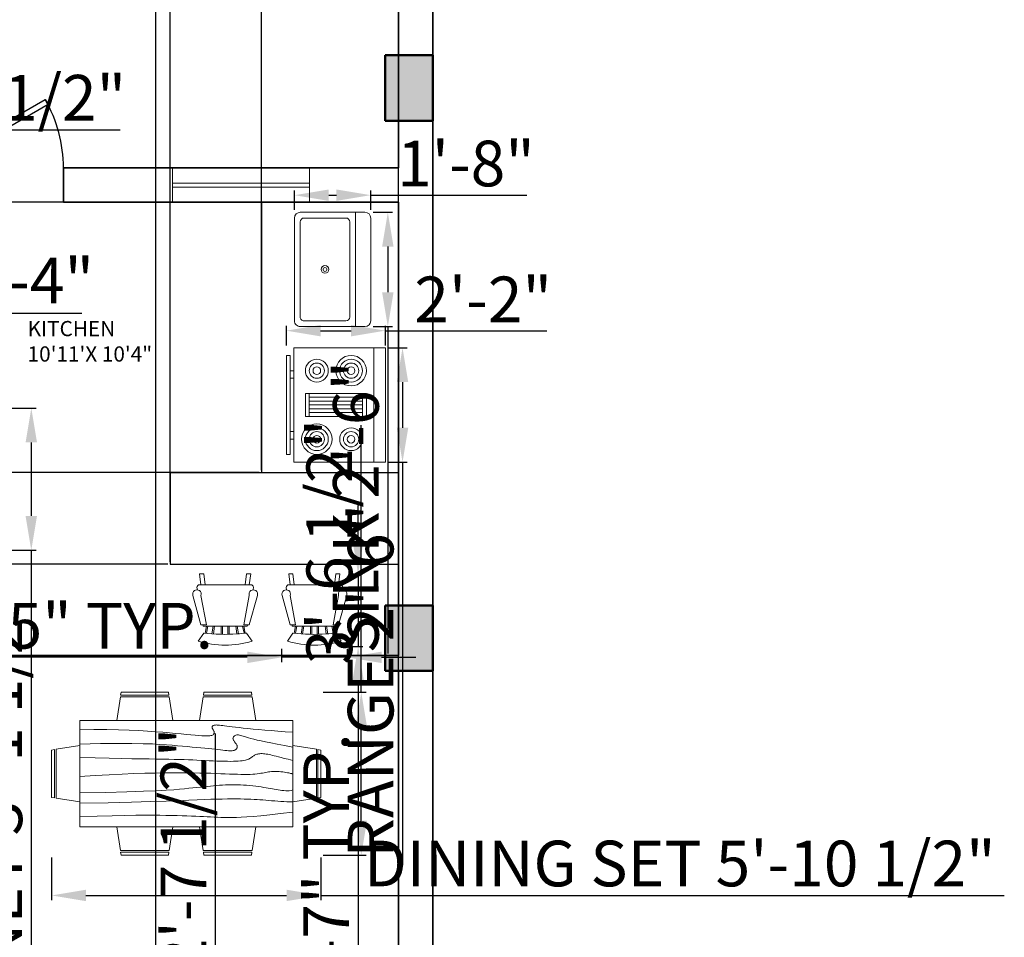
# Model space of a CAD drawing. Units: inches. Extents: x 1132 to 1713, y 3115 to 3781.
# Tile 3 of 4: x 1455 to 1713, y 3365 to 3606. Entities that reach past the tile are written whole.
import ezdxf

# ---------------------------------------------------------------- set-up
doc = ezdxf.new("R2010")
doc.units = ezdxf.units.IN
for name, color, linetype, lineweight in [('A-ANNO-DIMS', 2, 'Continuous', 18), ('A-AREA-IDEN', 7, 'Continuous', 18), ('A-COLS', 1, 'Continuous', 50), ('A-COLS-PATT', 252, 'Continuous', 13), ('A-DOOR', 3, 'Continuous', 25), ('A-EQPM', 8, 'Continuous', 18), ('A-FLOR-CASE', 30, 'Continuous', 25), ('A-FLOR-FIXT', 9, 'Continuous', 18), ('A-FURN', 8, 'Continuous', 18), ('A-GLAZ', 4, 'Continuous', 18), ('A-WALL', 7, 'Continuous', 35)]:
    doc.layers.add(name, color=color, linetype=linetype, lineweight=lineweight)
doc.styles.get("Standard").update_dxf_attribs({"font": 'arial.ttf'})
doc.dimstyles.new('ISO-25', dxfattribs={"dimtxt": 12, "dimasz": 9, "dimexe": 1.25, "dimexo": 0.625, "dimtad": 1, "dimdec": 0, "dimrnd": 2, "dimlunit": 3, "dimtxsty": 'Standard', "dimcen": 2.5, "dimadec": 0, "dimazin": 0, "dimtfac": 1, "dimtdec": 0, "dimtmove": 0, "dimatfit": 3, "dimfxl": 1, "dimarcsym": 0})

# ---------------------------------------------------------------- blocks, each defined once
blk = doc.blocks.new('*U2')
for p, q in [((0, 0), (0, -6)), ((40, 0), (40, -6))]:
    blk.add_line(p, q)
blk.add_lwpolyline([(0, 0), (34.64, 20), (35.52, 18.48), (0.87, -1.52)], close=True)
blk.add_arc((0, 0), 40, 0, 30)
blk = doc.blocks.new('Range-Oven - 30 in top')
for p, q in [((0, -3), (30, -3)), ((12, -6), (18, -6)), ((13, -20), (13, -6)), ((14, -6), (14, -20)), ((15, -20), (15, -6)), ((16, -6), (16, -20)), ((17, -20), (17, -6)), ((18, -20), (12, -20)), ((6, -24), (6, -25)), ((8, -25), (8, -24)), ((22, -25), (22, -24)), ((24, -24), (24, -25))]:
    blk.add_line(p, q)
for points in [[(0, -24), (0, 0), (30, 0), (30, -24)], [(12, -21), (12, -5), (18, -5), (18, -21)], [(2, -26), (2, -25), (28, -25), (28, -26)]]:
    blk.add_lwpolyline(points, close=True)
for centre, radius in [((6, -9), 4), ((6, -9), 3), ((6, -9), 2), ((24, -9), 3), ((24, -9), 2), ((6, -9), 1), ((24, -9), 1), ((6, -18), 3), ((24, -18), 4), ((24, -18), 3), ((6, -18), 2), ((6, -18), 1), ((24, -18), 2), ((24, -18), 1)]:
    blk.add_circle(centre, radius)
blk = doc.blocks.new('Sink-single - 30 in top')
blk.add_line((-15, -3.999996), (15, -3.999996))
for points in [[(-13.5, 0), (13.5, 0)], [(-15, -18.499996), (-15, -1.5)], [(15, -1.5), (15, -18.499996)], [(-13.5, -17.499996), (-13.5, -6.499996)], [(-12.5, -5.499996), (12.5, -5.499996)], [(13.5, -6.499996), (13.5, -17.499996)], [(13.5, -19.999996), (-13.5, -19.999996)], [(12.5, -18.499996), (-12.5, -18.499996)]]:
    blk.add_lwpolyline(points)
for radius in [1, 0.5]:
    blk.add_circle((0, -11.999996), radius)
for centre, radius, start, end in [((-13.5, -1.5), 1.5, 90, 180), ((13.5, -1.5), 1.5, 0, 90), ((-12.5, -6.499996), 1, 90, 180), ((12.5, -6.499996), 1, 0, 90), ((-12.5, -17.499996), 1, 180, 270), ((12.5, -17.499996), 1, 270, 0), ((-13.5, -18.499996), 1.5, 180, 270), ((13.5, -18.499996), 1.5, 270, 0)]:
    blk.add_arc(centre, radius, start, end)
blk = doc.blocks.new('Chair - Rocking')
for p, q in [((-8, -4.5), (-10, -1.5)), ((8, -4.5), (10, -1.5)), ((-8.23428, -6.99939), (-8.3093, -7.47958)), ((-8.23041, -7), (8.23915, -7)), ((-7.5, -4.5), (-7, -7)), ((-6.5, -7), (-7.02225, -4.43)), ((-4.5, -7), (-4.96674, -4.19951)), ((-4, -7), (-4.40532, -4.16272)), ((-1.5, -4.05012), (-1.5, -7)), ((-1, -7), (-1, -4.05012)), ((1, -7), (1, -4.04655)), ((1.5, -4.05012), (1.5, -7)), ((4, -7), (4.40187, -4.18694)), ((4.5, -7), (4.96761, -4.19437)), ((6.5, -7), (7, -4.4057)), ((7.5, -4.5), (7, -7)), ((8.31071, -7.48854), (8.23449, -7.00073)), ((-9, -7.5), (-12, -18.49999)), ((-7, -7.5), (-9, -7.5)), ((-9, -18.49999), (-7, -7.5)), ((7, -7.5), (9, -7.5)), ((9, -18.49999), (7, -7.5)), ((9, -7.5), (12, -18.49999)), ((-10.36644, -20.64523), (-10.5, -21.49999)), ((10.5, -21.49999), (10.3575, -20.58798)), ((-9, -22.49999), (-9.5, -26.49999)), ((0, -22.49999), (-9.5, -22.49999)), ((-8, -26.49999), (-7.5, -22.49999)), ((0, -22.49999), (9.5, -22.49999)), ((8, -26.49999), (7.5, -22.49999)), ((9, -22.49999), (9.5, -26.49999)), ((-9.5, -26.49999), (-8, -26.49999)), ((9.5, -26.49999), (8, -26.49999))]:
    blk.add_line(p, q)
for centre, radius, start, end in [((0, -34.08333), 34.08333, 72.93847, 107.0615), ((0, -68.25004), 64.25, 93.92211, 97.15267), ((0, -68.25004), 64.25, 82.84733, 93.92211), ((-10.5, -18.99999), 1.58114, 161.5651, 18.43495), ((-9.5, -21.49999), 1, 180, 270), ((10.5, -18.99999), 1.58114, 161.5651, 18.43495), ((9.5, -21.49999), 1, 270, 0)]:
    blk.add_arc(centre, radius, start, end)
blk = doc.blocks.new('Dining Set - 36 x 72 in.')
for p, q in [((-22, 27.5), (-22.1562, 26.50042)), ((-22, 27.5), (-6, 27.5)), ((-5.8437, 26.49966), (-6, 27.5)), ((6, 27.5), (5.8438, 26.50042)), ((6, 27.5), (22, 27.5)), ((22.1563, 26.49966), (22, 27.5)), ((-22.2343, 26.00059), (-23.4847, 17.99762)), ((-22.2304, 26), (-5.7608, 26)), ((-5.8416, 26.5), (-22.1534, 26.5)), ((-4.5152, 17.99762), (-5.7655, 25.99926)), ((5.7657, 26.00059), (4.5153, 17.99762)), ((5.7696, 26), (22.2392, 26)), ((22.1584, 26.5), (5.8466, 26.5)), ((23.4848, 17.99762), (22.2345, 25.99926)), ((36, 18), (-36, 18)), ((-36, 18), (-36, -18)), ((36, -18), (36, 18)), ((-45.5, 8), (-44.5004, 8.15617)), ((-45.5, 8), (-45.5, -8)), ((-44.5, -8.15843), (-44.5, 8.15338)), ((-44.0006, 8.23428), (-35.9976, 9.48474)), ((-44, 8.23041), (-44, -8.23915)), ((44.0006, 8.23428), (35.9976, 9.48474)), ((44, 8.23041), (44, -8.23915)), ((44.5, -8.15843), (44.5, 8.15338)), ((45.5, 8), (44.5005, 8.15617)), ((45.5, 8), (45.5, -8)), ((-44.4997, -8.15631), (-45.5, -8)), ((-35.9976, -9.48476), (-43.9993, -8.2345)), ((35.9976, -9.48476), (43.9993, -8.2345)), ((44.4997, -8.15631), (45.5, -8)), ((-36, -18), (36, -18)), ((-22.2343, -26.0006), (-23.4847, -17.99762)), ((-4.5152, -17.99762), (-5.7655, -25.99928)), ((5.7657, -26.0006), (4.5153, -17.99762)), ((23.4848, -17.99762), (22.2345, -25.99928)), ((-22.2304, -26), (-5.7608, -26)), ((-22, -27.5), (-22.1562, -26.50044)), ((-5.8416, -26.5), (-22.1534, -26.5)), ((-5.8437, -26.49967), (-6, -27.5)), ((5.7696, -26), (22.2392, -26)), ((6, -27.5), (5.8438, -26.50044)), ((22.1584, -26.5), (5.8466, -26.5)), ((22.1563, -26.49967), (22, -27.5)), ((-22, -27.5), (-6, -27.5)), ((6, -27.5), (22, -27.5))]:
    blk.add_line(p, q)
for points in [[(-36, 15), (-31.1772, 14.97754), (-26.8079, 14.91406), (-22.8538, 14.81543), (-19.276, 14.6875), (-16.0362, 14.53613), (-13.0957, 14.36718), (-10.4159, 14.18652), (-7.9583, 14), (-5.6904, 13.81315), (-3.6035, 13.63021), (-1.6954, 13.45508), (0.0365, 13.29166), (1.5945, 13.14388), (2.9811, 13.01562), (4.1988, 12.9108), (5.25, 12.83333), (6.1393, 12.78613), (6.8802, 12.76823), (7.4883, 12.77767), (7.9792, 12.8125), (8.3685, 12.87077), (8.6719, 12.95052), (8.9049, 13.0498), (9.0833, 13.16666), (9.2205, 13.29899), (9.3216, 13.44401), (9.3895, 13.59879), (9.4271, 13.76041), (9.4373, 13.92594), (9.4232, 14.09245), (9.3875, 14.257), (9.3333, 14.41666), (9.2638, 14.56917), (9.1836, 14.71484), (9.0975, 14.85465), (9.0104, 14.98958), (8.9272, 15.1206), (8.8529, 15.2487), (8.7922, 15.37483), (8.75, 15.5), (8.7305, 15.62467), (8.7344, 15.74739), (8.7617, 15.86621), (8.8125, 15.97916), (8.8867, 16.08431), (8.9844, 16.17968), (9.1055, 16.26334), (9.25, 16.33333), (9.4189, 16.38802), (9.6172, 16.42708), (9.8506, 16.45052), (10.125, 16.45833), (10.4463, 16.45052), (10.8203, 16.42708), (11.2529, 16.38802), (11.75, 16.33333), (12.3184, 16.26318), (12.9694, 16.17838), (13.7151, 16.07991), (14.5677, 15.96875), (15.5395, 15.84586), (16.6426, 15.71224), (17.8893, 15.56884), (19.2917, 15.41666), (20.859, 15.25667), (22.5879, 15.08984), (24.4721, 14.91715), (26.5052, 14.73958), (28.6809, 14.5581), (30.9929, 14.3737), (33.4347, 14.18733), (36, 14)], [(-36, 10), (-28.9766, 10.14274), (-23.1725, 10.20442), (-18.4241, 10.19775), (-14.5677, 10.13541), (-11.4399, 10.03011), (-8.877, 9.89453), (-6.7154, 9.74137), (-4.7917, 9.58333), (-2.9698, 9.43082), (-1.2246, 9.28515), (0.4415, 9.14534), (2.026, 9.01041), (3.5266, 8.87939), (4.9408, 8.7513), (6.266, 8.62516), (7.5, 8.5), (8.6411, 8.37549), (9.6914, 8.2539), (10.6538, 8.13818), (11.5312, 8.03125), (12.3267, 7.93603), (13.043, 7.85547), (13.6831, 7.79248), (14.25, 7.75), (14.7471, 7.7303), (15.1797, 7.73307), (15.5537, 7.75732), (15.875, 7.80208), (16.1494, 7.86637), (16.3828, 7.94922), (16.5811, 8.04964), (16.75, 8.16666), (16.8944, 8.29915), (17.0143, 8.44531), (17.1089, 8.60319), (17.1771, 8.77083), (17.218, 8.94629), (17.2305, 9.1276), (17.2137, 9.31282), (17.1667, 9.5), (17.0895, 9.6875), (16.987, 9.875), (16.8649, 10.0625), (16.7292, 10.25), (16.5856, 10.4375), (16.4401, 10.625), (16.2985, 10.8125), (16.1667, 11), (16.05, 11.18733), (15.9518, 11.3737), (15.8752, 11.5581), (15.8229, 11.73958), (15.798, 11.91715), (15.8034, 12.08984), (15.842, 12.25667), (15.9167, 12.41666), (16.0295, 12.56836), (16.1784, 12.70833), (16.3605, 12.83268), (16.5729, 12.9375), (16.8127, 13.01888), (17.0768, 13.07291), (17.3625, 13.0957), (17.6667, 13.08333), (17.9894, 13.03312), (18.3418, 12.94726), (18.7382, 12.82918), (19.1927, 12.68229), (19.7195, 12.51001), (20.3327, 12.31575), (21.0465, 12.10294), (21.875, 11.875), (22.8357, 11.63354), (23.959, 11.37304), (25.2786, 11.08618), (26.8282, 10.76562), (28.6414, 10.40405), (30.752, 9.99414), (33.1936, 9.52856), (36, 9)], [(-36, 5.5), (-30.7157, 5.3348), (-26.069, 5.20963), (-21.9946, 5.11767), (-18.4271, 5.05208), (-15.3009, 5.00602), (-12.5508, 4.97265), (-10.1112, 4.94515), (-7.9167, 4.91666), (-5.909, 4.88167), (-4.0586, 4.83984), (-2.3429, 4.79215), (-0.7396, 4.73958), (0.7739, 4.6831), (2.22, 4.6237), (3.6213, 4.56233), (5, 4.5), (6.373, 4.43782), (7.7344, 4.3776), (9.0723, 4.32129), (10.375, 4.27083), (11.6309, 4.22819), (12.8281, 4.19531), (13.9551, 4.17415), (15, 4.16666), (15.954, 4.17448), (16.819, 4.19791), (17.6001, 4.23698), (18.3021, 4.29166), (18.9299, 4.36198), (19.4883, 4.44791), (19.9823, 4.54948), (20.4167, 4.66666), (20.7969, 4.79899), (21.1302, 4.94401), (21.4245, 5.09879), (21.6875, 5.26041), (21.9271, 5.42594), (22.1511, 5.59245), (22.3672, 5.757), (22.5834, 5.91666), (22.8065, 6.06868), (23.0404, 6.21093), (23.2879, 6.34147), (23.5521, 6.45833), (23.8358, 6.55957), (24.142, 6.64323), (24.4735, 6.70735), (24.8334, 6.75), (25.2235, 6.76969), (25.642, 6.76692), (26.0858, 6.74267), (26.5521, 6.69791), (27.0379, 6.63362), (27.5404, 6.55078), (28.0565, 6.45036), (28.5834, 6.33333), (29.1242, 6.19987), (29.7071, 6.04687), (30.3661, 5.87044), (31.1354, 5.66666), (32.0493, 5.43164), (33.142, 5.16146), (34.4475, 4.85221), (36, 4.5)], [(-36, -1), (-30.7915, -0.6591), (-26.0195, -0.38216), (-21.6519, -0.16284), (-17.6563, 0.00521), (-14.0005, 0.12833), (-10.6523, 0.21289), (-7.5796, 0.26522), (-4.75, 0.29166), (-2.134, 0.29793), (0.2878, 0.28711), (2.5317, 0.26163), (4.6146, 0.22396), (6.5529, 0.17651), (8.3633, 0.12174), (10.0623, 0.06209), (11.6667, 0), (13.1899, -0.06201), (14.6341, -0.1211), (15.9982, -0.17432), (17.2813, -0.21875), (18.4823, -0.25147), (19.6003, -0.26953), (20.6343, -0.27002), (21.5834, -0.25), (22.4481, -0.20768), (23.2357, -0.14584), (23.9549, -0.06836), (24.6146, 0.02083), (25.2235, 0.11784), (25.7904, 0.21875), (26.3241, 0.31966), (26.8334, 0.41666), (27.3265, 0.50618), (27.8099, 0.58593), (28.2894, 0.65397), (28.7709, 0.70833), (29.2601, 0.74707), (29.763, 0.76823), (30.2855, 0.76985), (30.8334, 0.75), (31.4088, 0.70784), (31.9994, 0.64713), (32.589, 0.57275), (33.1615, 0.48958), (33.7008, 0.4025), (34.1908, 0.3164), (34.6153, 0.23616), (34.9584, 0.16666), (35.2099, 0.11165), (35.3848, 0.07031), (35.504, 0.04069), (35.5886, 0.02083), (35.6594, 0.00879), (35.7377, 0.0026), (35.8442, 0.00032), (36, 0)], [(-36, -6.5), (-27.1843, -6.31267), (-20.084, -6.1263), (-14.469, -5.9419), (-10.1094, -5.76042), (-6.7752, -5.58285), (-4.2363, -5.41016), (-2.2629, -5.24333), (-0.625, -5.08334), (0.8708, -4.93099), (2.2715, -4.78646), (3.5872, -4.64974), (4.8281, -4.52084), (6.0046, -4.39974), (7.127, -4.28646), (8.2053, -4.18099), (9.25, -4.08334), (10.2705, -3.99382), (11.2734, -3.91407), (12.2647, -3.84603), (13.25, -3.79167), (14.2354, -3.75293), (15.2266, -3.73177), (16.2295, -3.73015), (17.25, -3.75), (18.2912, -3.79248), (19.3451, -3.85547), (20.4009, -3.93604), (21.4479, -4.03125), (22.4754, -4.13819), (23.4727, -4.25391), (24.4289, -4.37549), (25.3334, -4.5), (26.1785, -4.62492), (26.9694, -4.74935), (27.7145, -4.87281), (28.4219, -4.99479), (29.1, -5.11483), (29.7572, -5.23242), (30.4016, -5.34709), (31.0417, -5.45834), (31.6837, -5.56437), (32.3262, -5.65821), (32.9658, -5.73153), (33.599, -5.77604), (34.2224, -5.78345), (34.8327, -5.74545), (35.4264, -5.65373), (36, -5.5)], [(-36, -10), (-26.4022, -9.81299), (-18.4675, -9.62891), (-11.9839, -9.45069), (-6.7396, -9.28125), (-2.5226, -9.12354), (0.8789, -8.98047), (3.6769, -8.85498), (6.0833, -8.75), (8.2767, -8.66765), (10.3021, -8.60677), (12.1712, -8.56543), (13.8958, -8.54167), (15.4876, -8.53353), (16.9583, -8.53907), (18.3197, -8.55632), (19.5834, -8.58334), (20.7616, -8.61841), (21.8685, -8.66081), (22.9188, -8.71004), (23.9271, -8.76563), (24.9081, -8.82707), (25.8763, -8.89388), (26.8465, -8.96558), (27.8334, -9.04167), (28.8474, -9.12118), (29.8828, -9.20117), (30.93, -9.27824), (31.9792, -9.34896), (33.0205, -9.40991), (34.0443, -9.45768), (35.0407, -9.48885), (36, -9.5)], [(-36, -14.5), (-30.0881, -14.33513), (-25.0332, -14.21224), (-20.7312, -14.12647), (-17.0781, -14.07292), (-13.97, -14.04671), (-11.3027, -14.04297), (-8.9724, -14.05681), (-6.875, -14.08334), (-4.9224, -14.11833), (-3.0905, -14.16016), (-1.3709, -14.20785), (0.2448, -14.26042), (1.7647, -14.3169), (3.1973, -14.3763), (4.5507, -14.43767), (5.8333, -14.5), (7.0554, -14.5621), (8.235, -14.62175), (9.3922, -14.67652), (10.5469, -14.72396), (11.7192, -14.76164), (12.929, -14.78711), (14.1965, -14.79794), (15.5417, -14.79167), (16.9933, -14.76424), (18.6152, -14.70508), (20.4804, -14.60197), (22.6615, -14.44271), (25.2312, -14.21509), (28.2624, -13.9069), (31.8277, -13.50594), (36, -13)]]:
    blk.add_lwpolyline(points)
blk = doc.blocks.new('WIN-36IN')
for p, q in [((-36, 0), (-36, 9)), ((-36, 9), (0, 9)), ((0, 9), (0, 0)), ((-36, 5), (0, 5)), ((0, 4), (-36, 4)), ((0, 0), (-36, 0))]:
    blk.add_line(p, q)
blk = doc.blocks.new('*D23')
at = {"layer": 'A-ANNO-DIMS', "color": 0, "lineweight": -2, "transparency": 16777216}
for p, q in [((1386.32, 3573.51), (1386.32, 3578.18)), ((1410.75, 3573.51), (1410.75, 3578.18)), ((1395.32, 3576.93), (1401.75, 3576.93)), ((1410.75, 3576.93), (1481.07, 3576.93))]:
    blk.add_line(p, q, dxfattribs=at)
at = {"layer": 'A-ANNO-DIMS', "color": 0, "transparency": 16777216}
for points in [[(1395.32, 3578.43), (1395.32, 3575.43), (1386.32, 3576.93)], [(1401.75, 3578.43), (1401.75, 3575.43), (1410.75, 3576.93)]]:
    blk.add_solid(points, dxfattribs=at)
at = {"layer": 'Defpoints', "color": 0, "transparency": 16777216}
for p in [(1410.75, 3576.93), (1386.32, 3572.88), (1410.75, 3572.88)]:
    blk.add_point(p, dxfattribs=at)
at = {"layer": 'A-ANNO-DIMS', "color": 0, "transparency": 16777216, "insert": (1450.41, 3583.76), "char_height": 12, "attachment_point": 5}
blk.add_mtext('2\'-0 1/2"', dxfattribs=at)
blk = doc.blocks.new('*D24')
at = {"layer": 'A-ANNO-DIMS', "color": 0, "lineweight": -2, "transparency": 16777216}
for p, q in [((1543.52, 3469.28), (1543.52, 3478.28)), ((1541.29, 3460.28), (1544.77, 3460.28)), ((1543.52, 3460.28), (1543.52, 3441.25)), ((1541.29, 3441.25), (1544.77, 3441.25)), ((1543.52, 3432.25), (1543.52, 3273.09))]:
    blk.add_line(p, q, dxfattribs=at)
at = {"layer": 'A-ANNO-DIMS', "color": 0, "transparency": 16777216}
for points in [[(1542.02, 3469.28), (1545.02, 3469.28), (1543.52, 3460.28)], [(1542.02, 3432.25), (1545.02, 3432.25), (1543.52, 3441.25)]]:
    blk.add_solid(points, dxfattribs=at)
at = {"layer": 'Defpoints', "color": 0, "transparency": 16777216}
for p in [(1540.66, 3460.28), (1540.66, 3441.25), (1543.52, 3441.25)]:
    blk.add_point(p, dxfattribs=at)
at = {"layer": 'A-ANNO-DIMS', "color": 0, "transparency": 16777216, "insert": (1536.68, 3348.17), "char_height": 12, "attachment_point": 5, "rotation": 90}
blk.add_mtext('ROCKER 1\'-7" TYP.', dxfattribs=at)
blk = doc.blocks.new('*D25')
at = {"layer": 'A-ANNO-DIMS', "color": 0, "lineweight": -2, "transparency": 16777216}
for p, q in [((1514.43, 3438.39), (1432.17, 3438.39)), ((1523.43, 3440.62), (1523.43, 3437.14)), ((1540.66, 3438.39), (1523.43, 3438.39)), ((1540.66, 3440.62), (1540.66, 3437.14)), ((1549.66, 3438.39), (1558.66, 3438.39))]:
    blk.add_line(p, q, dxfattribs=at)
at = {"layer": 'A-ANNO-DIMS', "color": 0, "transparency": 16777216}
for points in [[(1514.43, 3439.89), (1514.43, 3436.89), (1523.43, 3438.39)], [(1549.66, 3439.89), (1549.66, 3436.89), (1540.66, 3438.39)]]:
    blk.add_solid(points, dxfattribs=at)
at = {"layer": 'Defpoints', "color": 0, "transparency": 16777216}
for p in [(1523.43, 3441.25), (1540.66, 3441.25), (1523.43, 3438.39)]:
    blk.add_point(p, dxfattribs=at)
at = {"layer": 'A-ANNO-DIMS', "color": 0, "transparency": 16777216, "insert": (1468.8, 3445.14), "char_height": 12, "attachment_point": 5}
blk.add_mtext('1\'-5" TYP.', dxfattribs=at)
blk = doc.blocks.new('*D31')
at = {"layer": 'A-ANNO-DIMS', "color": 0, "lineweight": -2, "transparency": 16777216}
for p, q in [((1506.04, 3348.05), (1506.04, 3418.37)), ((1498.97, 3348.05), (1507.29, 3348.05)), ((1506.04, 3325.7), (1506.04, 3339.05)), ((1498.97, 3316.7), (1507.29, 3316.7))]:
    blk.add_line(p, q, dxfattribs=at)
at = {"layer": 'A-ANNO-DIMS', "color": 0, "transparency": 16777216}
for points in [[(1504.54, 3339.05), (1507.54, 3339.05), (1506.04, 3348.05)], [(1504.54, 3325.7), (1507.54, 3325.7), (1506.04, 3316.7)]]:
    blk.add_solid(points, dxfattribs=at)
at = {"layer": 'Defpoints', "color": 0, "transparency": 16777216}
for p in [(1498.35, 3348.05), (1506.04, 3348.05), (1498.35, 3316.7)]:
    blk.add_point(p, dxfattribs=at)
at = {"layer": 'A-ANNO-DIMS', "color": 0, "transparency": 16777216, "insert": (1499.21, 3387.71), "char_height": 12, "attachment_point": 5, "rotation": 90}
blk.add_mtext('2\'-7 1/2"', dxfattribs=at)
blk = doc.blocks.new('*D34')
at = {"layer": 'A-ANNO-DIMS', "color": 0, "lineweight": -2, "transparency": 16777216}
for p, q in [((1551.3, 3519.66), (1556.43, 3519.66)), ((1555.18, 3510.66), (1555.18, 3498.66)), ((1551.3, 3489.66), (1556.43, 3489.66)), ((1555.18, 3489.66), (1555.18, 3383.86))]:
    blk.add_line(p, q, dxfattribs=at)
at = {"layer": 'A-ANNO-DIMS', "color": 0, "transparency": 16777216}
for points in [[(1553.68, 3510.66), (1556.68, 3510.66), (1555.18, 3519.66)], [(1553.68, 3498.66), (1556.68, 3498.66), (1555.18, 3489.66)]]:
    blk.add_solid(points, dxfattribs=at)
at = {"layer": 'Defpoints', "color": 0, "transparency": 16777216}
for p in [(1550.68, 3519.66), (1550.68, 3489.66), (1555.18, 3489.66)]:
    blk.add_point(p, dxfattribs=at)
at = {"layer": 'A-ANNO-DIMS', "color": 0, "transparency": 16777216, "insert": (1548.35, 3432.26), "char_height": 12, "attachment_point": 5, "rotation": 90}
blk.add_mtext('RANGE 2\'-6"', dxfattribs=at)
blk = doc.blocks.new('*D35')
at = {"layer": 'A-ANNO-DIMS', "color": 0, "lineweight": -2, "transparency": 16777216}
for p, q in [((1524.68, 3520.28), (1524.68, 3525.41)), ((1533.68, 3524.16), (1541.68, 3524.16)), ((1550.68, 3520.28), (1550.68, 3525.41)), ((1550.68, 3524.16), (1593.03, 3524.16))]:
    blk.add_line(p, q, dxfattribs=at)
at = {"layer": 'A-ANNO-DIMS', "color": 0, "transparency": 16777216}
for points in [[(1533.68, 3525.66), (1533.68, 3522.66), (1524.68, 3524.16)], [(1541.68, 3525.66), (1541.68, 3522.66), (1550.68, 3524.16)]]:
    blk.add_solid(points, dxfattribs=at)
at = {"layer": 'Defpoints', "color": 0, "transparency": 16777216}
for p in [(1550.68, 3524.16), (1524.68, 3519.66), (1550.68, 3519.66)]:
    blk.add_point(p, dxfattribs=at)
at = {"layer": 'A-ANNO-DIMS', "color": 0, "transparency": 16777216, "insert": (1576.35, 3530.81), "char_height": 12, "attachment_point": 5}
blk.add_mtext('2\'-2"', dxfattribs=at)
blk = doc.blocks.new('*D40')
at = {"layer": 'A-ANNO-DIMS', "color": 0, "lineweight": -2, "transparency": 16777216}
for p, q in [((1452.73, 3503.82), (1458.96, 3503.82)), ((1457.71, 3494.82), (1457.71, 3475.51)), ((1452.73, 3466.51), (1458.96, 3466.51)), ((1457.71, 3466.51), (1457.71, 3319.22))]:
    blk.add_line(p, q, dxfattribs=at)
at = {"layer": 'A-ANNO-DIMS', "color": 0, "transparency": 16777216}
for points in [[(1456.21, 3494.82), (1459.21, 3494.82), (1457.71, 3503.82)], [(1456.21, 3475.51), (1459.21, 3475.51), (1457.71, 3466.51)]]:
    blk.add_solid(points, dxfattribs=at)
at = {"layer": 'Defpoints', "color": 0, "transparency": 16777216}
for p in [(1452.11, 3503.82), (1452.11, 3466.51), (1457.71, 3466.51)]:
    blk.add_point(p, dxfattribs=at)
at = {"layer": 'A-ANNO-DIMS', "color": 0, "transparency": 16777216, "insert": (1450.87, 3388.36), "char_height": 12, "attachment_point": 5, "rotation": 90}
blk.add_mtext('CABINET 3\'-1 1/2"', dxfattribs=at)
blk = doc.blocks.new('*D42')
at = {"layer": 'A-ANNO-DIMS', "color": 0, "lineweight": -2, "transparency": 16777216}
for p, q in [((1547.44, 3555.24), (1552.57, 3555.24)), ((1551.32, 3546.24), (1551.32, 3534.24)), ((1547.44, 3525.24), (1552.57, 3525.24)), ((1551.32, 3525.24), (1551.32, 3439.37))]:
    blk.add_line(p, q, dxfattribs=at)
at = {"layer": 'A-ANNO-DIMS', "color": 0, "transparency": 16777216}
for points in [[(1549.82, 3546.24), (1552.82, 3546.24), (1551.32, 3555.24)], [(1549.82, 3534.24), (1552.82, 3534.24), (1551.32, 3525.24)]]:
    blk.add_solid(points, dxfattribs=at)
at = {"layer": 'Defpoints', "color": 0, "transparency": 16777216}
for p in [(1546.82, 3555.24), (1546.82, 3525.24), (1551.32, 3525.24)]:
    blk.add_point(p, dxfattribs=at)
at = {"layer": 'A-ANNO-DIMS', "color": 0, "transparency": 16777216, "insert": (1544.49, 3477.81), "char_height": 12, "attachment_point": 5, "rotation": 90}
blk.add_mtext('SINK 2\'-6"', dxfattribs=at)
blk = doc.blocks.new('*D43')
at = {"layer": 'A-ANNO-DIMS', "color": 0, "lineweight": -2, "transparency": 16777216}
for p, q in [((1526.82, 3555.87), (1526.82, 3560.99)), ((1535.82, 3559.74), (1537.82, 3559.74)), ((1546.82, 3555.87), (1546.82, 3560.99)), ((1546.82, 3559.74), (1587.84, 3559.74))]:
    blk.add_line(p, q, dxfattribs=at)
at = {"layer": 'A-ANNO-DIMS', "color": 0, "transparency": 16777216}
for points in [[(1535.82, 3561.24), (1535.82, 3558.24), (1526.82, 3559.74)], [(1537.82, 3561.24), (1537.82, 3558.24), (1546.82, 3559.74)]]:
    blk.add_solid(points, dxfattribs=at)
at = {"layer": 'Defpoints', "color": 0, "transparency": 16777216}
for p in [(1546.82, 3559.74), (1526.82, 3555.24), (1546.82, 3555.24)]:
    blk.add_point(p, dxfattribs=at)
at = {"layer": 'A-ANNO-DIMS', "color": 0, "transparency": 16777216, "insert": (1571.83, 3566.5), "char_height": 12, "attachment_point": 5}
blk.add_mtext('1\'-8"', dxfattribs=at)
blk = doc.blocks.new('*D44')
at = {"layer": 'A-ANNO-DIMS', "color": 0, "lineweight": -2, "transparency": 16777216}
for p, q in [((1463.04, 3385.85), (1463.04, 3374.62)), ((1533.74, 3385.85), (1533.74, 3374.62)), ((1472.04, 3375.87), (1524.74, 3375.87)), ((1533.74, 3375.87), (1713.17, 3375.87))]:
    blk.add_line(p, q, dxfattribs=at)
at = {"layer": 'A-ANNO-DIMS', "color": 0, "transparency": 16777216}
for points in [[(1472.04, 3377.37), (1472.04, 3374.37), (1463.04, 3375.87)], [(1524.74, 3377.37), (1524.74, 3374.37), (1533.74, 3375.87)]]:
    blk.add_solid(points, dxfattribs=at)
at = {"layer": 'Defpoints', "color": 0, "transparency": 16777216}
for p in [(1463.04, 3386.48), (1533.74, 3386.48), (1533.74, 3375.87)]:
    blk.add_point(p, dxfattribs=at)
at = {"layer": 'A-ANNO-DIMS', "color": 0, "transparency": 16777216, "insert": (1627.96, 3382.7), "char_height": 12, "attachment_point": 5}
blk.add_mtext('DINING SET 5\'-10 1/2"', dxfattribs=at)
blk = doc.blocks.new('*D45')
at = {"layer": 'A-ANNO-DIMS', "color": 0, "lineweight": -2, "transparency": 16777216}
for p, q in [((1544.35, 3429.21), (1544.35, 3499.31)), ((1534.37, 3429.21), (1545.6, 3429.21)), ((1544.35, 3395.48), (1544.35, 3420.21)), ((1534.37, 3386.48), (1545.6, 3386.48))]:
    blk.add_line(p, q, dxfattribs=at)
at = {"layer": 'A-ANNO-DIMS', "color": 0, "transparency": 16777216}
for points in [[(1542.85, 3420.21), (1545.85, 3420.21), (1544.35, 3429.21)], [(1542.85, 3395.48), (1545.85, 3395.48), (1544.35, 3386.48)]]:
    blk.add_solid(points, dxfattribs=at)
at = {"layer": 'Defpoints', "color": 0, "transparency": 16777216}
for p in [(1533.74, 3429.21), (1544.35, 3429.21), (1533.74, 3386.48)]:
    blk.add_point(p, dxfattribs=at)
at = {"layer": 'A-ANNO-DIMS', "color": 0, "transparency": 16777216, "insert": (1537.51, 3468.76), "char_height": 12, "attachment_point": 5, "rotation": 90}
blk.add_mtext('3\'-6 1/2"', dxfattribs=at)
blk = doc.blocks.new('*D50')
at = {"layer": 'A-ANNO-DIMS', "color": 0, "lineweight": -2, "transparency": 16777216}
for p, q in [((1490.38, 3260.74), (1490.38, 3701.81)), ((1554.16, 3217.5), (1554.16, 3701.81)), ((1499.38, 3700.56), (1545.16, 3700.56))]:
    blk.add_line(p, q, dxfattribs=at)
at = {"layer": 'A-ANNO-DIMS', "color": 0, "transparency": 16777216}
for points in [[(1499.38, 3702.06), (1499.38, 3699.06), (1490.38, 3700.56)], [(1545.16, 3702.06), (1545.16, 3699.06), (1554.16, 3700.56)]]:
    blk.add_solid(points, dxfattribs=at)
at = {"layer": 'Defpoints', "color": 0, "transparency": 16777216}
for p in [(1554.16, 3700.56), (1490.38, 3260.12), (1554.16, 3216.88)]:
    blk.add_point(p, dxfattribs=at)
at = {"layer": 'A-ANNO-DIMS', "color": 0, "transparency": 16777216, "insert": (1522.27, 3707.29), "char_height": 12, "attachment_point": 5}
blk.add_mtext('5\'-4"', dxfattribs=at)
blk = doc.blocks.new('*D55')
at = {"layer": 'A-ANNO-DIMS', "color": 0, "lineweight": -2, "transparency": 16777216}
for p, q in [((1494.16, 3463.5), (1494.16, 3701.81)), ((1554.16, 3463.5), (1554.16, 3701.81)), ((1503.16, 3700.56), (1545.16, 3700.56))]:
    blk.add_line(p, q, dxfattribs=at)
at = {"layer": 'A-ANNO-DIMS', "color": 0, "transparency": 16777216}
for points in [[(1503.16, 3702.06), (1503.16, 3699.06), (1494.16, 3700.56)], [(1545.16, 3702.06), (1545.16, 3699.06), (1554.16, 3700.56)]]:
    blk.add_solid(points, dxfattribs=at)
at = {"layer": 'Defpoints', "color": 0, "transparency": 16777216}
for p in [(1554.16, 3700.56), (1494.16, 3462.88), (1554.16, 3462.88)]:
    blk.add_point(p, dxfattribs=at)
at = {"layer": 'A-ANNO-DIMS', "color": 0, "transparency": 16777216, "insert": (1524.16, 3707.31), "char_height": 12, "attachment_point": 5}
blk.add_mtext('5\'-0"', dxfattribs=at)
blk = doc.blocks.new('*D56')
at = {"layer": 'A-ANNO-DIMS', "color": 0, "lineweight": -2, "transparency": 16777216}
for p, q in [((1238.49, 3486.88), (1238.49, 3529.23)), ((1493.53, 3486.88), (1237.24, 3486.88)), ((1238.49, 3471.88), (1238.49, 3477.88)), ((1493.53, 3462.88), (1237.24, 3462.88))]:
    blk.add_line(p, q, dxfattribs=at)
at = {"layer": 'A-ANNO-DIMS', "color": 0, "transparency": 16777216}
for points in [[(1236.99, 3477.88), (1239.99, 3477.88), (1238.49, 3486.88)], [(1236.99, 3471.88), (1239.99, 3471.88), (1238.49, 3462.88)]]:
    blk.add_solid(points, dxfattribs=at)
at = {"layer": 'Defpoints', "color": 0, "transparency": 16777216}
for p in [(1238.49, 3486.88), (1494.16, 3486.88), (1494.16, 3462.88)]:
    blk.add_point(p, dxfattribs=at)
at = {"layer": 'A-ANNO-DIMS', "color": 0, "transparency": 16777216, "insert": (1231.73, 3512.55), "char_height": 12, "attachment_point": 5, "rotation": 90}
blk.add_mtext('2\'-0"', dxfattribs=at)
blk = doc.blocks.new('*D57')
at = {"layer": 'A-ANNO-DIMS', "color": 0, "lineweight": -2, "transparency": 16777216}
for p, q in [((1517.53, 3557.88), (1237.24, 3557.88)), ((1238.49, 3495.88), (1238.49, 3548.88)), ((1517.53, 3486.88), (1237.24, 3486.88))]:
    blk.add_line(p, q, dxfattribs=at)
at = {"layer": 'A-ANNO-DIMS', "color": 0, "transparency": 16777216}
for points in [[(1236.99, 3548.88), (1239.99, 3548.88), (1238.49, 3557.88)], [(1236.99, 3495.88), (1239.99, 3495.88), (1238.49, 3486.88)]]:
    blk.add_solid(points, dxfattribs=at)
at = {"layer": 'Defpoints', "color": 0, "transparency": 16777216}
for p in [(1238.49, 3557.88), (1518.16, 3557.88), (1518.16, 3486.88)]:
    blk.add_point(p, dxfattribs=at)
at = {"layer": 'A-ANNO-DIMS', "color": 0, "transparency": 16777216, "insert": (1231.73, 3522.38), "char_height": 12, "attachment_point": 5, "rotation": 90}
blk.add_mtext('5\'-11"', dxfattribs=at)
blk = doc.blocks.new('*D58')
at = {"layer": 'A-ANNO-DIMS', "color": 0, "lineweight": -2, "transparency": 16777216}
for p, q in [((1494.16, 3487.5), (1494.16, 3701.81)), ((1518.16, 3487.5), (1518.16, 3701.81)), ((1503.16, 3700.56), (1509.16, 3700.56)), ((1518.16, 3700.56), (1560.51, 3700.56))]:
    blk.add_line(p, q, dxfattribs=at)
at = {"layer": 'A-ANNO-DIMS', "color": 0, "transparency": 16777216}
for points in [[(1503.16, 3702.06), (1503.16, 3699.06), (1494.16, 3700.56)], [(1509.16, 3702.06), (1509.16, 3699.06), (1518.16, 3700.56)]]:
    blk.add_solid(points, dxfattribs=at)
at = {"layer": 'Defpoints', "color": 0, "transparency": 16777216}
for p in [(1518.16, 3700.56), (1494.16, 3486.88), (1518.16, 3486.88)]:
    blk.add_point(p, dxfattribs=at)
at = {"layer": 'A-ANNO-DIMS', "color": 0, "transparency": 16777216, "insert": (1543.84, 3707.31), "char_height": 12, "attachment_point": 5}
blk.add_mtext('2\'-0"', dxfattribs=at)
blk = doc.blocks.new('*D59')
at = {"layer": 'A-ANNO-DIMS', "color": 0, "lineweight": -2, "transparency": 16777216}
for p, q in [((1381.6, 3528.66), (1372.6, 3528.66)), ((1390.6, 3528.66), (1406.81, 3528.66)), ((1471.02, 3528.66), (1415.81, 3528.66))]:
    blk.add_line(p, q, dxfattribs=at)
at = {"layer": 'A-ANNO-DIMS', "color": 0, "transparency": 16777216}
for points in [[(1381.6, 3530.16), (1381.6, 3527.16), (1390.6, 3528.66)], [(1415.81, 3530.16), (1415.81, 3527.16), (1406.81, 3528.66)]]:
    blk.add_solid(points, dxfattribs=at)
at = {"layer": 'Defpoints', "color": 0, "transparency": 16777216}
for p in [(1390.6, 3528.66), (1406.81, 3528.66)]:
    blk.add_point(p, dxfattribs=at)
at = {"layer": 'A-ANNO-DIMS', "color": 0, "transparency": 16777216, "insert": (1447.92, 3535.75), "char_height": 12, "attachment_point": 5, "rotation": 0.002}
blk.add_mtext('∅1\'-4"', dxfattribs=at)

msp = doc.modelspace()

# ---------------------------------------------------------------- hatches: boundary and pattern name
at = {"layer": 'A-COLS-PATT'}
h = msp.add_hatch(color=256, dxfattribs=at)
h.dxf.hatch_style = 1
h.paths.add_polyline_path([(1550.64, 3579.3), (1554.16, 3579.3), (1554.16, 3596.47), (1550.64, 3596.47)])
h = msp.add_hatch(color=256, dxfattribs=at)
h.dxf.hatch_style = 1
h.paths.add_polyline_path([(1563.14, 3596.47), (1554.16, 3596.47), (1554.16, 3579.3), (1563.14, 3579.3)])
h = msp.add_hatch(color=256, dxfattribs=at)
h.dxf.hatch_style = 1
h.paths.add_polyline_path([(1554.16, 3438.88), (1550.65, 3438.88), (1550.65, 3434.88), (1554.16, 3434.88), (1563.15, 3434.87), (1563.15, 3452.04), (1554.16, 3452.04)])
h = msp.add_hatch(color=256, dxfattribs=at)
h.dxf.hatch_style = 1
h.paths.add_polyline_path([(1554.16, 3452.04), (1550.65, 3452.04), (1550.65, 3438.88), (1554.16, 3438.88)])

# ---------------------------------------------------------------- linework, layer by layer
at = {"layer": 'A-COLS'}
for p, q in [((1550.64, 3596.47), (1563.14, 3596.47)), ((1550.64, 3579.3), (1550.64, 3596.47)), ((1563.14, 3596.47), (1563.14, 3579.3)), ((1563.14, 3579.3), (1550.64, 3579.3)), ((1550.65, 3452.04), (1563.15, 3452.04)), ((1550.65, 3434.87), (1550.65, 3452.04)), ((1563.15, 3452.04), (1563.15, 3434.87)), ((1563.15, 3434.87), (1550.65, 3434.87))]:
    msp.add_line(p, q, dxfattribs=at)
at = {"layer": 'A-FLOR-CASE'}
for p, q in [((1518.16, 3557.88), (1518.16, 3486.88)), ((1494.16, 3486.88), (1554.16, 3486.88)), ((1494.16, 3486.88), (1494.16, 3462.88)), ((1494.16, 3462.88), (1554.16, 3462.88))]:
    msp.add_line(p, q, dxfattribs=at)
at = {"layer": 'A-WALL'}
for p, q in [((1554.16, 3661.88), (1554.16, 3566.88)), ((1466.16, 3557.88), (1466.16, 3566.88)), ((1466.16, 3566.88), (1554.16, 3566.88)), ((1466.16, 3557.88), (1554.16, 3557.88)), ((1554.16, 3557.88), (1554.16, 3438.88)), ((1425.16, 3438.88), (1554.16, 3438.88)), ((1554.16, 3434.88), (1554.16, 3216.88))]:
    msp.add_line(p, q, dxfattribs=at)
msp.add_lwpolyline([(1268.16, 3670.88), (1563.16, 3670.88), (1563.16, 3145.88), (1268.16, 3145.88)], close=True, dxfattribs=at)

# ---------------------------------------------------------------- block references
at = {"layer": 'A-DOOR', "xscale": 0.9, "yscale": 0.9, "zscale": 0.9}
msp.add_blockref('*U2', (1430.16, 3566.88), dxfattribs=at)
at = {"layer": 'A-EQPM', "rotation": 270}
msp.add_blockref('Range-Oven - 30 in top', (1550.68, 3519.66), dxfattribs=at)
at = {"layer": 'A-FLOR-FIXT', "rotation": 270}
msp.add_blockref('Sink-single - 30 in top', (1546.82, 3540.24), dxfattribs=at)
at = {"layer": 'A-FURN', "xscale": 0.7051131052241644, "yscale": 0.7051131052241644, "zscale": 0.7051131052241644, "rotation": 180}
for p in [(1508.61, 3441.6), (1532.05, 3441.6)]:
    msp.add_blockref('Chair - Rocking', p, dxfattribs=at)
at = {"layer": 'A-FURN', "xscale": 0.7769976174684975, "yscale": 0.7769976174684975, "zscale": 0.7769976174684975}
msp.add_blockref('Dining Set - 36 x 72 in.', (1498.39, 3407.84), dxfattribs=at)
at = {"layer": 'A-GLAZ'}
msp.add_blockref('WIN-36IN', (1530.75, 3557.88), dxfattribs=at)

# ---------------------------------------------------------------- texts
at = {"layer": 'A-AREA-IDEN', "insert": (1456.74, 3526.71), "char_height": 4, "attachment_point": 1}
msp.add_mtext_dynamic_manual_height_columns('{\\fArial|b1|i0|c0|p34;KITCHEN\\P10\'11\'X 10\'4"}', width=83.7568, gutter_width=12.5, heights=[54.87], dxfattribs=at)

# ---------------------------------------------------------------- dimensions: what is measured, and where the dimension line sits
at = {"layer": 'A-ANNO-DIMS'}
for base, p1, p2, picture, middle in [((1554.16, 3700.56), (1490.38, 3260.12), (1554.16, 3216.88), '*D50', (1522.27, 3707.29)), ((1554.16, 3700.56), (1494.16, 3462.88), (1554.16, 3462.88), '*D55', (1524.16, 3707.31)), ((1518.16, 3700.56), (1494.16, 3486.88), (1518.16, 3486.88), '*D58', (1543.84, 3707.31)), ((1410.75, 3576.93), (1386.32, 3572.88), (1410.75, 3572.88), '*D23', (1450.41, 3583.76)), ((1546.82, 3559.74), (1526.82, 3555.24), (1546.82, 3555.24), '*D43', (1571.83, 3566.5)), ((1550.68, 3524.16), (1524.68, 3519.66), (1550.68, 3519.66), '*D35', (1576.35, 3530.81))]:
    dim = msp.add_linear_dim(base=base, p1=p1, p2=p2, dimstyle='ISO-25', override={"dimdec": 1, "dimlfac": 1, "dimrnd": 0, "dimzin": 1, "dimdsep": 46, "dimlunit": 4, "dimfrac": 2}, dxfattribs=at)
    dim.commit()
    dim.dimension.update_dxf_attribs({"geometry": picture, "text_midpoint": middle})
for base, p1, p2, picture, middle in [((1238.49, 3557.88), (1518.16, 3486.88), (1518.16, 3557.88), '*D57', (1231.73, 3522.38)), ((1238.49, 3486.88), (1494.16, 3462.88), (1494.16, 3486.88), '*D56', (1231.73, 3512.55)), ((1544.35, 3429.21), (1533.74, 3386.48), (1533.74, 3429.21), '*D45', (1537.51, 3468.76)), ((1506.0429, 3348.0538), (1498.3462, 3316.6969), (1498.3462, 3348.0538), '*D31', (1499.2133, 3387.7115))]:
    dim = msp.add_linear_dim(base=base, p1=p1, p2=p2, angle=90, dimstyle='ISO-25', override={"dimdec": 1, "dimlfac": 1, "dimrnd": 0, "dimzin": 1, "dimdsep": 46, "dimlunit": 4, "dimfrac": 2}, dxfattribs=at)
    dim.commit()
    dim.dimension.update_dxf_attribs({"geometry": picture, "text_midpoint": middle})
for base, p1, p2, angle, text, picture, middle in [((1551.32, 3525.24), (1546.82, 3555.24), (1546.82, 3525.24), 270, 'SINK <>', '*D42', (1544.49, 3477.81)), ((1555.18, 3489.66), (1550.68, 3519.66), (1550.68, 3489.66), 270, 'RANGE <>', '*D34', (1548.35, 3432.26)), ((1457.71, 3466.51), (1452.11, 3503.82), (1452.11, 3466.51), 270, 'CABINET <>', '*D40', (1450.87, 3388.36)), ((1543.52, 3441.25), (1540.66, 3460.28), (1540.66, 3441.25), 270, 'ROCKER <> TYP.', '*D24', (1536.68, 3348.17)), ((1523.43, 3438.39), (1540.66, 3441.25), (1523.43, 3441.25), 180, '<> TYP.', '*D25', (1468.8, 3445.14))]:
    dim = msp.add_linear_dim(base=base, p1=p1, p2=p2, angle=angle, text=text, dimstyle='ISO-25', override={"dimdec": 1, "dimlfac": 1, "dimrnd": 0, "dimzin": 1, "dimdsep": 46, "dimlunit": 4, "dimfrac": 2}, dxfattribs=at)
    dim.commit()
    dim.dimension.update_dxf_attribs({"geometry": picture, "text_midpoint": middle})
dim = msp.add_diameter_dim_2p(p1=(1390.6, 3528.66), p2=(1406.81, 3528.66), dimstyle='ISO-25', override={"dimdec": 1, "dimlfac": 1, "dimrnd": 0, "dimzin": 1, "dimdsep": 46, "dimlunit": 4, "dimfrac": 2}, dxfattribs=at)
dim.commit()
dim.dimension.update_dxf_attribs({"geometry": '*D59', "text_midpoint": (1447.92, 3528.66), "dimtype": 163})
dim = msp.add_linear_dim(base=(1533.74, 3375.87), p1=(1463.04, 3386.48), p2=(1533.74, 3386.48), text='DINING SET <>', dimstyle='ISO-25', override={"dimdec": 1, "dimlfac": 1, "dimrnd": 0, "dimzin": 1, "dimdsep": 46, "dimlunit": 4, "dimfrac": 2}, dxfattribs=at)
dim.commit()
dim.dimension.update_dxf_attribs({"geometry": '*D44', "text_midpoint": (1627.96, 3382.7)})

doc.saveas('drawing.dxf')
